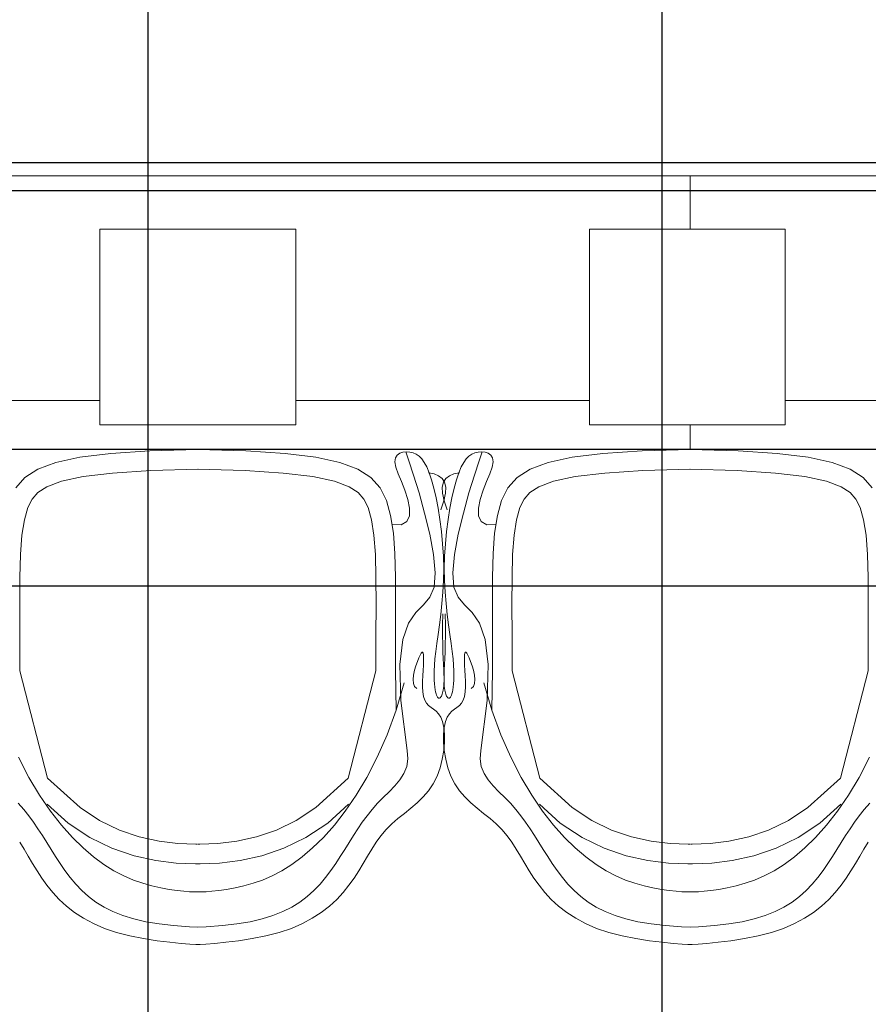
# Model space of a CAD drawing. Units: inches. Extents: x 1454 to 2136, y 626 to 1213.
# Tile 9 of 23: x 1620 to 1654, y 1062 to 1101. Entities that reach past the tile are written whole.
import ezdxf

# ---------------------------------------------------------------- set-up
doc = ezdxf.new("R2010")
doc.units = ezdxf.units.IN
doc.header["$MEASUREMENT"] = 0
for name, color, linetype, lineweight in [('A-ANNO-DIMS', 2, 'Continuous', 18), ('A-FURN-PATT', 252, 'Continuous', 13), ('conference', 41, 'Continuous', 18)]:
    doc.layers.add(name, color=color, linetype=linetype, lineweight=lineweight)
doc.styles.get("Standard").update_dxf_attribs({"font": 'arial.ttf'})
doc.dimstyles.get("Standard").update_dxf_attribs({"dimtxt": 4, "dimasz": 0.18, "dimexe": 0.18, "dimexo": 0.0625, "dimgap": 0.09, "dimtad": 0, "dimtih": 1, "dimtoh": 1, "dimdec": 0, "dimrnd": 6, "dimzin": 0, "dimdsep": 46, "dimlunit": 3, "dimtxsty": 'Standard', "dimcen": 0.09, "dimadec": 0, "dimazin": 0, "dimtfac": 1, "dimtdec": 0, "dimtofl": 0, "dimtmove": 0, "dimatfit": 3, "dimfxl": 1, "dimtolj": 1, "dimtzin": 0, "dimarcsym": 0})

# ---------------------------------------------------------------- blocks, each defined once
blk = doc.blocks.new('ОГ52_на12персон_стол2800х900')
for p, q in [((-1220.7, -341.4), (1220.7, -341.4)), ((-0.6, -341.4), (-0.6, -395.7)), ((-603.4, -595.7), (-603.4, -395.7)), ((-603.4, -395.7), (-403.4, -395.7)), ((-403.4, -395.7), (-403.4, -595.7)), ((-103.4, -595.7), (-103.4, -395.7)), ((-103.4, -395.7), (96.6, -395.7)), ((96.6, -395.7), (96.6, -595.7)), ((-903.4, -570.7), (-603.4, -570.7)), ((-403.4, -570.7), (-103.4, -570.7)), ((96.6, -570.7), (403.4, -570.7)), ((-403.4, -595.7), (-603.4, -595.7)), ((96.6, -595.7), (-103.4, -595.7)), ((-0.6, -595.7), (-0.6, -620.7)), ((-1300, -620.7), (1300, -620.7)), ((-592.3, -624.8), (-552.5, -622.2)), ((-552.5, -622.2), (-503.4, -620.7)), ((-454.3, -622.2), (-503.4, -620.7)), ((-414.4, -624.8), (-454.3, -622.2)), ((-293.9, -623.5), (-290.4, -623.2)), ((-287.8, -632.3), (-290.9, -623.2)), ((-290.4, -623.2), (-286.9, -623.5)), ((-213.6, -623.2), (-217.1, -623.5)), ((-216.2, -632.3), (-213.1, -623.2)), ((-210.1, -623.5), (-213.6, -623.2)), ((-89.6, -624.8), (-49.7, -622.2)), ((-49.7, -622.2), (-0.6, -620.7)), ((48.5, -622.2), (-0.6, -620.7)), ((88.3, -624.8), (48.5, -622.2)), ((-648.5, -633.9), (-624, -628.7)), ((-624, -628.7), (-592.3, -624.8)), ((-382.8, -628.7), (-414.4, -624.8)), ((-358.3, -633.9), (-382.8, -628.7)), ((-302.1, -633.5), (-301.5, -629.4)), ((-301.5, -629.4), (-299.7, -626.5)), ((-299.7, -626.5), (-297.1, -624.6)), ((-297.1, -624.6), (-293.9, -623.5)), ((-283.1, -646.8), (-287.8, -632.3)), ((-286.9, -623.5), (-283.6, -624.2)), ((-283.6, -624.2), (-280.4, -625.5)), ((-280.4, -625.5), (-277.5, -627.4)), ((-277.5, -627.4), (-274.7, -630.2)), ((-274.7, -630.2), (-272.1, -633.9)), ((-229.3, -630.2), (-231.9, -633.9)), ((-226.5, -627.4), (-229.3, -630.2)), ((-223.6, -625.5), (-226.5, -627.4)), ((-220.4, -624.2), (-223.6, -625.5)), ((-220.9, -646.8), (-216.2, -632.3)), ((-217.1, -623.5), (-220.4, -624.2)), ((-206.9, -624.6), (-210.1, -623.5)), ((-204.3, -626.5), (-206.9, -624.6)), ((-202.5, -629.4), (-204.3, -626.5)), ((-201.9, -633.5), (-202.5, -629.4)), ((-145.7, -633.9), (-121.2, -628.7)), ((-121.2, -628.7), (-89.6, -624.8)), ((120, -628.7), (88.3, -624.8)), ((144.5, -633.9), (120, -628.7)), ((-680.2, -649.4), (-666.8, -640.7)), ((-666.8, -640.7), (-648.5, -633.9)), ((-590.5, -644.8), (-551.5, -642.2)), ((-551.5, -642.2), (-502.7, -640.7)), ((-455.2, -642.2), (-504, -640.7)), ((-416.3, -644.8), (-455.2, -642.2)), ((-339.9, -640.7), (-358.3, -633.9)), ((-326.6, -649.4), (-339.9, -640.7)), ((-301.3, -638.8), (-302.1, -633.5)), ((-298.9, -645.6), (-301.3, -638.8)), ((-272.1, -633.9), (-269.5, -638.6)), ((-269.5, -638.6), (-267.1, -644.5)), ((-234.5, -638.6), (-236.9, -644.5)), ((-231.9, -633.9), (-234.5, -638.6)), ((-205.1, -645.6), (-202.7, -638.8)), ((-202.7, -638.8), (-201.9, -633.5)), ((-177.4, -649.4), (-164.1, -640.7)), ((-164.1, -640.7), (-145.7, -633.9)), ((-87.8, -644.8), (-48.8, -642.2)), ((-48.8, -642.2), (0, -640.7)), ((47.5, -642.2), (-1.3, -640.7)), ((86.5, -644.8), (47.5, -642.2)), ((162.8, -640.7), (144.5, -633.9)), ((176.2, -649.4), (162.8, -640.7)), ((-689.5, -660), (-680.2, -649.4)), ((-657.8, -658.7), (-642.8, -653.1)), ((-642.8, -653.1), (-620.7, -648.4)), ((-620.7, -648.4), (-590.5, -644.8)), ((-386.1, -648.4), (-416.3, -644.8)), ((-363.9, -653.1), (-386.1, -648.4)), ((-349, -658.7), (-363.9, -653.1)), ((-317.3, -660), (-326.6, -649.4)), ((-298.9, -645.6), (-295.5, -653.4)), ((-295.5, -653.4), (-292, -662.3)), ((-277.5, -665.1), (-283.1, -646.8)), ((-262.2, -645.6), (-267.7, -644.5)), ((-267.1, -644.5), (-264.7, -651.7)), ((-264.7, -651.7), (-262.3, -660.3)), ((-257.6, -647.6), (-262.2, -645.6)), ((-254, -650.4), (-257.6, -647.6)), ((-251.5, -654.2), (-254, -650.4)), ((-252.5, -654.2), (-250, -650.4)), ((-250, -650.4), (-246.4, -647.6)), ((-246.4, -647.6), (-241.8, -645.6)), ((-241.8, -645.6), (-236.3, -644.5)), ((-239.3, -651.7), (-241.7, -660.3)), ((-236.9, -644.5), (-239.3, -651.7)), ((-226.5, -665.1), (-220.9, -646.8)), ((-208.5, -653.4), (-212, -662.3)), ((-205.1, -645.6), (-208.5, -653.4)), ((-186.7, -660), (-177.4, -649.4)), ((-155.1, -658.7), (-140.1, -653.1)), ((-140.1, -653.1), (-117.9, -648.4)), ((-117.9, -648.4), (-87.8, -644.8)), ((116.7, -648.4), (86.5, -644.8)), ((138.8, -653.1), (116.7, -648.4)), ((153.8, -658.7), (138.8, -653.1)), ((185.5, -660), (176.2, -649.4)), ((-666.9, -664.7), (-657.8, -658.7)), ((-339.8, -664.7), (-349, -658.7)), ((-310.9, -672.9), (-317.3, -660)), ((-292, -662.3), (-289.1, -671.7)), ((-262.3, -660.3), (-260.1, -670)), ((-253.8, -659.2), (-252.5, -654.2)), ((-253.6, -665.5), (-253.8, -659.2)), ((-250.2, -659.2), (-251.5, -654.2)), ((-250.4, -665.5), (-250.2, -659.2)), ((-241.7, -660.3), (-243.9, -670)), ((-212, -662.3), (-214.9, -671.7)), ((-193.1, -672.9), (-186.7, -660)), ((-164.2, -664.7), (-155.1, -658.7)), ((162.9, -664.7), (153.8, -658.7)), ((-677.1, -680.1), (-672.7, -671.3)), ((-672.7, -671.3), (-666.9, -664.7)), ((-334, -671.3), (-339.8, -664.7)), ((-329.6, -680.1), (-334, -671.3)), ((-306.5, -688.1), (-310.9, -672.9)), ((-289.1, -671.7), (-287.3, -680.7)), ((-271.8, -685.8), (-277.5, -665.1)), ((-260.1, -670), (-258, -680.8)), ((-255.4, -682.4), (-252.1, -673.2)), ((-251.9, -673.2), (-253.6, -665.5)), ((-252.1, -673.2), (-250.4, -665.5)), ((-248.6, -682.4), (-251.9, -673.2)), ((-243.9, -670), (-246, -680.8)), ((-232.2, -685.8), (-226.5, -665.1)), ((-214.9, -671.7), (-216.7, -680.7)), ((-197.5, -688.1), (-193.1, -672.9)), ((-174.4, -680.1), (-170, -671.3)), ((-170, -671.3), (-164.2, -664.7)), ((168.7, -671.3), (162.9, -664.7)), ((173.1, -680.1), (168.7, -671.3)), ((-680.6, -692.4), (-677.1, -680.1)), ((-326.1, -692.4), (-329.6, -680.1)), ((-287.3, -680.7), (-287.3, -688.5)), ((-258, -680.8), (-256.2, -692.3)), ((-246, -680.8), (-247.8, -692.3)), ((-216.7, -680.7), (-216.7, -688.5)), ((-177.9, -692.4), (-174.4, -680.1)), ((176.6, -692.4), (173.1, -680.1)), ((-683.1, -708.3), (-680.6, -692.4)), ((-323.6, -708.3), (-326.1, -692.4)), ((-303.7, -706), (-306.5, -688.1)), ((-287.3, -688.5), (-289.9, -694.3)), ((-266.6, -707.3), (-271.8, -685.8)), ((-256.2, -692.3), (-254.6, -704.4)), ((-247.8, -692.3), (-249.4, -704.4)), ((-237.4, -707.3), (-232.2, -685.8)), ((-216.7, -688.5), (-214.1, -694.3)), ((-200.3, -706), (-197.5, -688.1)), ((-180.4, -708.3), (-177.9, -692.4)), ((179.1, -708.3), (176.6, -692.4)), ((-295.6, -697.5), (-305.1, -697.1)), ((-289.9, -694.3), (-295.6, -697.5)), ((-214.1, -694.3), (-208.4, -697.5)), ((-208.4, -697.5), (-198.9, -697.1)), ((-684.6, -728), (-683.1, -708.3)), ((-322.1, -728), (-323.6, -708.3)), ((-302.2, -726.9), (-303.7, -706)), ((-262.8, -728.1), (-266.6, -707.3)), ((-254.6, -704.4), (-253.4, -716.9)), ((-249.4, -704.4), (-250.6, -716.9)), ((-241.2, -728.1), (-237.4, -707.3)), ((-201.8, -726.9), (-200.3, -706)), ((-181.9, -728), (-180.4, -708.3)), ((180.6, -728), (179.1, -708.3)), ((-253.4, -716.9), (-252.6, -729.5)), ((-250.6, -716.9), (-251.4, -729.5)), ((-685.3, -751.4), (-684.6, -728)), ((-321.5, -751.4), (-322.1, -728)), ((-301.5, -751.1), (-302.2, -726.9)), ((-261.1, -746.6), (-262.8, -728.1)), ((-252.6, -729.5), (-252.3, -742.1)), ((-251.4, -729.5), (-251.7, -742.1)), ((-242.9, -746.6), (-241.2, -728.1)), ((-202.5, -751.1), (-201.8, -726.9)), ((-182.5, -751.4), (-181.9, -728)), ((181.2, -751.4), (180.6, -728)), ((-252.3, -742.1), (-252.5, -754.5)), ((-251.7, -742.1), (-251.5, -754.5)), ((-685.4, -778.9), (-685.3, -751.4)), ((-321.4, -778.9), (-321.5, -751.4)), ((-301.4, -778.9), (-301.5, -751.1)), ((-262.2, -761.4), (-261.1, -746.6)), ((-241.8, -761.4), (-242.9, -746.6)), ((-202.6, -778.9), (-202.5, -751.1)), ((-182.6, -778.9), (-182.5, -751.4)), ((181.4, -778.9), (181.2, -751.4)), ((-266.5, -771.5), (-262.2, -761.4)), ((-252.5, -754.5), (-253.1, -766.5)), ((-251.5, -754.5), (-250.9, -766.5)), ((-237.5, -771.5), (-241.8, -761.4)), ((-273.1, -779.2), (-266.5, -771.5)), ((-253.1, -766.5), (-254.1, -778.1)), ((-250.9, -766.5), (-249.9, -778.1)), ((-230.9, -779.2), (-237.5, -771.5)), ((-685.3, -810.5), (-685.4, -778.9)), ((-321.5, -810.5), (-321.4, -778.9)), ((-301.5, -810.6), (-301.4, -778.9)), ((-280.7, -787), (-273.1, -779.2)), ((-254.1, -778.1), (-255.4, -789.2)), ((-249.9, -778.1), (-248.7, -789.2)), ((-223.3, -787), (-230.9, -779.2)), ((-202.5, -810.6), (-202.6, -778.9)), ((-182.5, -810.5), (-182.6, -778.9)), ((181.3, -810.5), (181.4, -778.9)), ((-288.1, -798), (-280.7, -787)), ((-255.4, -789.2), (-256.7, -799.7)), ((-253.5, -800.2), (-253.3, -788.5)), ((-250.5, -800.2), (-250.7, -788.5)), ((-248.7, -789.2), (-247.3, -799.7)), ((-215.9, -798), (-223.3, -787)), ((-294, -814.7), (-288.1, -798)), ((-256.7, -799.7), (-258, -809.6)), ((-253.4, -810.5), (-253.5, -800.2)), ((-250.6, -810.5), (-250.5, -800.2)), ((-247.3, -799.7), (-246, -809.6)), ((-210.1, -814.7), (-215.9, -798)), ((-685.3, -846.6), (-685.3, -810.5)), ((-321.5, -846.6), (-321.5, -810.5)), ((-301.5, -846.4), (-301.5, -810.6)), ((-258, -809.6), (-259.3, -818.7)), ((-253.3, -819.6), (-253.4, -810.5)), ((-250.7, -819.6), (-250.6, -810.5)), ((-246, -809.6), (-244.7, -818.7)), ((-202.5, -846.4), (-202.5, -810.6)), ((-182.5, -846.6), (-182.5, -810.5)), ((181.3, -846.6), (181.3, -810.5)), ((-297, -840.1), (-294, -814.7)), ((-259.3, -818.7), (-260.4, -827)), ((-253.1, -827.5), (-253.3, -819.6)), ((-250.9, -827.5), (-250.7, -819.6)), ((-244.7, -818.7), (-243.6, -827)), ((-207, -840.1), (-210.1, -814.7)), ((-279.2, -837.1), (-277.7, -833.4)), ((-277.7, -833.4), (-276.4, -830.6)), ((-276.4, -830.6), (-275.3, -828.7)), ((-275.3, -828.7), (-274.4, -827.8)), ((-274.4, -827.8), (-273.8, -827.7)), ((-273.8, -827.7), (-273.3, -828.6)), ((-273.3, -828.6), (-272.9, -830.5)), ((-272.9, -830.5), (-272.8, -833.2)), ((-272.8, -833.2), (-272.9, -836.7)), ((-260.4, -827), (-261.2, -834.4)), ((-252.8, -834.3), (-253.1, -827.5)), ((-252.5, -840.3), (-252.8, -834.3)), ((-251.5, -840.3), (-251.2, -834.3)), ((-251.2, -834.3), (-250.9, -827.5)), ((-243.6, -827), (-242.8, -834.4)), ((-231.1, -830.5), (-231.2, -833.2)), ((-231.2, -833.2), (-231.1, -836.7)), ((-230.7, -828.6), (-231.1, -830.5)), ((-230.3, -827.7), (-230.7, -828.6)), ((-229.6, -827.8), (-230.3, -827.7)), ((-228.7, -828.7), (-229.6, -827.8)), ((-227.6, -830.6), (-228.7, -828.7)), ((-226.3, -833.4), (-227.6, -830.6)), ((-224.8, -837.1), (-226.3, -833.4)), ((-296, -876.9), (-297, -840.1)), ((-282, -846.2), (-280.7, -841.5)), ((-280.7, -841.5), (-279.2, -837.1)), ((-273.1, -841.2), (-273.4, -846.2)), ((-272.9, -836.7), (-273.1, -841.2)), ((-261.7, -841), (-262, -846.8)), ((-261.2, -834.4), (-261.7, -841)), ((-252.3, -845.4), (-252.5, -840.3)), ((-251.7, -845.4), (-251.5, -840.3)), ((-242.8, -834.4), (-242.3, -841)), ((-242.3, -841), (-242, -846.8)), ((-231.1, -836.7), (-230.9, -841.2)), ((-230.9, -841.2), (-230.6, -846.2)), ((-223.3, -841.5), (-224.8, -837.1)), ((-222, -846.2), (-223.3, -841.5)), ((-208, -876.9), (-207, -840.1)), ((-657, -956.4), (-685.3, -846.6)), ((-349.8, -956.4), (-321.5, -846.6)), ((-301, -886.8), (-301.5, -846.4)), ((-283.5, -855.5), (-283, -851)), ((-283, -851), (-282, -846.2)), ((-273.6, -851.7), (-273.8, -857.3)), ((-273.4, -846.2), (-273.6, -851.7)), ((-262, -846.8), (-262, -851.9)), ((-262, -851.9), (-261.9, -856.3)), ((-252.1, -849.8), (-252.3, -845.4)), ((-252, -853.7), (-252.1, -849.8)), ((-252, -853.7), (-251.9, -849.8)), ((-252, -857), (-252, -853.7)), ((-252, -857), (-252, -853.7)), ((-251.9, -849.8), (-251.7, -845.4)), ((-242, -851.9), (-242.1, -856.3)), ((-242, -846.8), (-242, -851.9)), ((-230.6, -846.2), (-230.4, -851.7)), ((-230.4, -851.7), (-230.2, -857.3)), ((-221, -851), (-222, -846.2)), ((-220.5, -855.5), (-221, -851)), ((-203, -886.8), (-202.5, -846.4)), ((-154.2, -956.4), (-182.5, -846.6)), ((153, -956.4), (181.3, -846.6)), ((-292.7, -859), (-301, -886.8)), ((-283.2, -859.6), (-283.5, -855.5)), ((-282.1, -862.7), (-283.2, -859.6)), ((-279.9, -864.8), (-282.1, -862.7)), ((-273.8, -857.3), (-273.8, -862.9)), ((-273.8, -862.9), (-273.5, -868.2)), ((-261.9, -856.3), (-261.7, -860.1)), ((-261.7, -860.1), (-261.4, -863.3)), ((-261.4, -863.3), (-261, -866)), ((-252.8, -866.3), (-252.5, -864.5)), ((-252.5, -864.5), (-252.3, -862.4)), ((-252.3, -862.4), (-252.1, -859.9)), ((-252.1, -859.9), (-252, -857)), ((-251.9, -859.9), (-252, -857)), ((-251.7, -862.4), (-251.9, -859.9)), ((-251.5, -864.5), (-251.7, -862.4)), ((-251.2, -866.3), (-251.5, -864.5)), ((-242.6, -863.3), (-243, -866)), ((-242.3, -860.1), (-242.6, -863.3)), ((-242.1, -856.3), (-242.3, -860.1)), ((-230.2, -862.9), (-230.5, -868.2)), ((-230.2, -857.3), (-230.2, -862.9)), ((-224.1, -864.8), (-221.9, -862.7)), ((-221.9, -862.7), (-220.8, -859.6)), ((-220.8, -859.6), (-220.5, -855.5)), ((-211.3, -859), (-203, -886.8)), ((-273.5, -868.2), (-272.8, -872.9)), ((-272.8, -872.9), (-271.6, -876.8)), ((-261, -866), (-260.6, -868.3)), ((-260.6, -868.3), (-260.1, -870.2)), ((-260.1, -870.2), (-259.6, -871.7)), ((-259.6, -871.7), (-259.1, -872.9)), ((-259.1, -872.9), (-258.6, -873.7)), ((-258.6, -873.7), (-258.1, -874.3)), ((-258.1, -874.3), (-257.6, -874.6)), ((-256.5, -874.6), (-256, -874.3)), ((-256, -874.3), (-255.6, -873.9)), ((-255.6, -873.9), (-255.1, -873.3)), ((-255.1, -873.3), (-254.7, -872.5)), ((-254.7, -872.5), (-254.2, -871.6)), ((-254.2, -871.6), (-253.8, -870.5)), ((-253.8, -870.5), (-253.5, -869.2)), ((-253.5, -869.2), (-253.1, -867.9)), ((-253.1, -867.9), (-252.8, -866.3)), ((-250.9, -867.9), (-251.2, -866.3)), ((-250.6, -869.2), (-250.9, -867.9)), ((-250.2, -870.5), (-250.6, -869.2)), ((-249.8, -871.6), (-250.2, -870.5)), ((-249.3, -872.5), (-249.8, -871.6)), ((-248.9, -873.3), (-249.3, -872.5)), ((-248.4, -873.9), (-248.9, -873.3)), ((-248, -874.3), (-248.4, -873.9)), ((-247.5, -874.6), (-248, -874.3)), ((-245.9, -874.3), (-246.4, -874.6)), ((-245.4, -873.7), (-245.9, -874.3)), ((-244.9, -872.9), (-245.4, -873.7)), ((-244.4, -871.7), (-244.9, -872.9)), ((-243.9, -870.2), (-244.4, -871.7)), ((-243.4, -868.3), (-243.9, -870.2)), ((-243, -866), (-243.4, -868.3)), ((-231.2, -872.9), (-232.4, -876.8)), ((-230.5, -868.2), (-231.2, -872.9)), ((-289.6, -927.9), (-296, -876.9)), ((-271.6, -876.8), (-269.8, -879.9)), ((-269.8, -879.9), (-267.7, -882.2)), ((-267.7, -882.2), (-265.2, -884.1)), ((-265.2, -884.1), (-262.6, -886)), ((-257.6, -874.6), (-257, -874.7)), ((-257, -874.7), (-256.5, -874.6)), ((-247, -874.7), (-247.5, -874.6)), ((-246.4, -874.6), (-247, -874.7)), ((-238.8, -884.1), (-241.4, -886)), ((-236.3, -882.2), (-238.8, -884.1)), ((-234.2, -879.9), (-236.3, -882.2)), ((-232.4, -876.8), (-234.2, -879.9)), ((-214.4, -927.9), (-208, -876.9)), ((-301, -886.8), (-310.2, -912.1)), ((-262.6, -886), (-260, -888)), ((-260, -888), (-257.5, -890.6)), ((-257.5, -890.6), (-255.3, -894)), ((-255.3, -894), (-253.5, -898.6)), ((-248.7, -894), (-250.5, -898.6)), ((-246.5, -890.6), (-248.7, -894)), ((-244, -888), (-246.5, -890.6)), ((-241.4, -886), (-244, -888)), ((-203, -886.8), (-193.8, -912.1)), ((-253.5, -898.6), (-252.3, -904.5)), ((-251.7, -904.5), (-252.4, -911.6)), ((-252.3, -904.5), (-251.6, -911.6)), ((-250.5, -898.6), (-251.7, -904.5)), ((-310.2, -912.1), (-320.1, -934.9)), ((-252.4, -911.6), (-252.4, -919.5)), ((-251.6, -911.6), (-251.6, -919.5)), ((-193.8, -912.1), (-183.9, -934.9)), ((-252.4, -919.5), (-251.7, -928)), ((-251.6, -919.5), (-252.3, -928)), ((-289.6, -927.9), (-288.8, -936.5)), ((-252.3, -928), (-253.8, -936.8)), ((-251.7, -928), (-250.2, -936.8)), ((-214.4, -927.9), (-215.2, -936.5)), ((-686.6, -934.9), (-676.1, -955.5)), ((-320.1, -934.9), (-330.7, -955.5)), ((-290, -944.3), (-292.9, -951.4)), ((-288.8, -936.5), (-290, -944.3)), ((-253.8, -936.8), (-256, -945.6)), ((-250.2, -936.8), (-248, -945.6)), ((-215.2, -936.5), (-214, -944.3)), ((-214, -944.3), (-211.1, -951.4)), ((-183.9, -934.9), (-173.3, -955.5)), ((182.6, -934.9), (172.1, -955.5)), ((-292.9, -951.4), (-297.1, -958)), ((-259.1, -954.1), (-263, -962)), ((-256, -945.6), (-259.1, -954.1)), ((-248, -945.6), (-244.9, -954.1)), ((-244.9, -954.1), (-241, -962)), ((-211.1, -951.4), (-206.9, -958)), ((-676.1, -955.5), (-665.2, -973.8)), ((-657, -956.4), (-623.7, -986.3)), ((-349.8, -956.4), (-383, -986.3)), ((-330.7, -955.5), (-341.6, -973.8)), ((-302.3, -964.1), (-308, -970.1)), ((-297.1, -958), (-302.3, -964.1)), ((-263, -962), (-267.8, -969.1)), ((-241, -962), (-236.2, -969.1)), ((-206.9, -958), (-201.7, -964.1)), ((-201.7, -964.1), (-196, -970.1)), ((-173.3, -955.5), (-162.4, -973.8)), ((-154.2, -956.4), (-121, -986.3)), ((153, -956.4), (119.7, -986.3)), ((172.1, -955.5), (161.2, -973.8)), ((-665.2, -973.8), (-654, -990)), ((-341.6, -973.8), (-352.8, -990)), ((-308, -970.1), (-314.1, -976)), ((-267.8, -969.1), (-273.4, -975.5)), ((-236.2, -969.1), (-230.6, -975.5)), ((-196, -970.1), (-190, -976)), ((-162.4, -973.8), (-151.3, -990)), ((161.2, -973.8), (150, -990)), ((-686.8, -982), (-681.3, -988.2)), ((-657.3, -983), (-636, -1002.1)), ((-349.4, -983), (-370.7, -1002.1)), ((-320, -982), (-325.5, -988.2)), ((-314.1, -976), (-320, -982)), ((-279.5, -981.4), (-285.9, -986.9)), ((-273.4, -975.5), (-279.5, -981.4)), ((-230.6, -975.5), (-224.5, -981.4)), ((-224.5, -981.4), (-218.1, -986.9)), ((-190, -976), (-184, -982)), ((-184, -982), (-178.5, -988.2)), ((-154.6, -983), (-133.3, -1002.1)), ((153.3, -983), (132, -1002.1)), ((182.8, -982), (177.3, -988.2)), ((-681.3, -988.2), (-676.1, -994.6)), ((-676.1, -994.6), (-671.3, -1001.3)), ((-654, -990), (-642.7, -1004.3)), ((-623.7, -986.3), (-603.8, -999.5)), ((-383, -986.3), (-402.9, -999.5)), ((-352.8, -990), (-364, -1004.3)), ((-330.6, -994.6), (-335.5, -1001.3)), ((-325.5, -988.2), (-330.6, -994.6)), ((-292.5, -992.3), (-299, -997.6)), ((-285.9, -986.9), (-292.5, -992.3)), ((-218.1, -986.9), (-211.5, -992.3)), ((-211.5, -992.3), (-205, -997.6)), ((-178.5, -988.2), (-173.4, -994.6)), ((-173.4, -994.6), (-168.6, -1001.3)), ((-151.3, -990), (-140, -1004.3)), ((-121, -986.3), (-101.1, -999.5)), ((119.7, -986.3), (99.8, -999.5)), ((150, -990), (138.7, -1004.3)), ((172.1, -994.6), (167.3, -1001.3)), ((177.3, -988.2), (172.1, -994.6)), ((-671.3, -1001.3), (-666.7, -1008.1)), ((-642.7, -1004.3), (-631.5, -1016.8)), ((-636, -1002.1), (-613.8, -1016.9)), ((-603.8, -999.5), (-583.6, -1009.3)), ((-402.9, -999.5), (-423.2, -1009.3)), ((-370.7, -1002.1), (-393, -1016.9)), ((-364, -1004.3), (-375.2, -1016.8)), ((-335.5, -1001.3), (-340.1, -1008.1)), ((-305.3, -1003), (-311.2, -1008.8)), ((-299, -997.6), (-305.3, -1003)), ((-205, -997.6), (-198.7, -1003)), ((-198.7, -1003), (-192.8, -1008.8)), ((-168.6, -1001.3), (-163.9, -1008.1)), ((-140, -1004.3), (-128.8, -1016.8)), ((-133.3, -1002.1), (-111, -1016.9)), ((-101.1, -999.5), (-80.8, -1009.3)), ((99.8, -999.5), (79.6, -1009.3)), ((132, -1002.1), (109.8, -1016.9)), ((138.7, -1004.3), (127.5, -1016.8)), ((167.3, -1001.3), (162.7, -1008.1)), ((-666.7, -1008.1), (-662.2, -1015)), ((-662.2, -1015), (-657.8, -1022.1)), ((-583.6, -1009.3), (-563.2, -1016.2)), ((-423.2, -1009.3), (-443.5, -1016.2)), ((-344.5, -1015), (-348.9, -1022.1)), ((-340.1, -1008.1), (-344.5, -1015)), ((-316.5, -1015.1), (-321.3, -1021.7)), ((-311.2, -1008.8), (-316.5, -1015.1)), ((-192.8, -1008.8), (-187.5, -1015.1)), ((-187.5, -1015.1), (-182.7, -1021.7)), ((-163.9, -1008.1), (-159.5, -1015)), ((-159.5, -1015), (-155.1, -1022.1)), ((-80.8, -1009.3), (-60.5, -1016.2)), ((79.6, -1009.3), (59.2, -1016.2)), ((158.2, -1015), (153.8, -1022.1)), ((162.7, -1008.1), (158.2, -1015)), ((-685.4, -1021.7), (-680.9, -1028.7)), ((-657.8, -1022.1), (-653.4, -1029.2)), ((-631.5, -1016.8), (-620.6, -1027.5)), ((-613.8, -1016.9), (-591.2, -1027.9)), ((-563.2, -1016.2), (-543.1, -1020.6)), ((-543.1, -1020.6), (-523.8, -1023)), ((-523.8, -1023), (-505.5, -1023.8)), ((-505.5, -1023.8), (-503.8, -1023.8)), ((-501.3, -1023.8), (-503, -1023.8)), ((-483, -1023), (-501.3, -1023.8)), ((-463.6, -1020.6), (-483, -1023)), ((-443.5, -1016.2), (-463.6, -1020.6)), ((-393, -1016.9), (-415.6, -1027.9)), ((-375.2, -1016.8), (-386.2, -1027.5)), ((-348.9, -1022.1), (-353.4, -1029.2)), ((-321.3, -1021.7), (-325.8, -1028.7)), ((-182.7, -1021.7), (-178.2, -1028.7)), ((-155.1, -1022.1), (-150.6, -1029.2)), ((-128.8, -1016.8), (-117.9, -1027.5)), ((-111, -1016.9), (-88.4, -1027.9)), ((-60.5, -1016.2), (-40.4, -1020.6)), ((-40.4, -1020.6), (-21, -1023)), ((-21, -1023), (-2.7, -1023.8)), ((-2.7, -1023.8), (-1, -1023.8)), ((1.5, -1023.8), (-0.2, -1023.8)), ((19.7, -1023), (1.5, -1023.8)), ((39.1, -1020.6), (19.7, -1023)), ((59.2, -1016.2), (39.1, -1020.6)), ((109.8, -1016.9), (87.2, -1027.9)), ((127.5, -1016.8), (116.6, -1027.5)), ((153.8, -1022.1), (149.4, -1029.2)), ((181.4, -1021.7), (176.9, -1028.7)), ((-680.9, -1028.7), (-676.6, -1035.9)), ((-653.4, -1029.2), (-648.8, -1036.4)), ((-620.6, -1027.5), (-609.9, -1036.7)), ((-591.2, -1027.9), (-568.6, -1035.5)), ((-415.6, -1027.9), (-438.1, -1035.5)), ((-386.2, -1027.5), (-396.9, -1036.7)), ((-353.4, -1029.2), (-357.9, -1036.4)), ((-325.8, -1028.7), (-330.2, -1035.9)), ((-178.2, -1028.7), (-173.9, -1035.9)), ((-150.6, -1029.2), (-146.1, -1036.4)), ((-117.9, -1027.5), (-107.1, -1036.7)), ((-88.4, -1027.9), (-65.9, -1035.5)), ((87.2, -1027.9), (64.6, -1035.5)), ((116.6, -1027.5), (105.9, -1036.7)), ((149.4, -1029.2), (144.8, -1036.4)), ((176.9, -1028.7), (172.6, -1035.9)), ((-676.6, -1035.9), (-672.2, -1043.3)), ((-672.2, -1043.3), (-667.7, -1050.8)), ((-648.8, -1036.4), (-644.1, -1043.6)), ((-644.1, -1043.6), (-639.2, -1050.7)), ((-609.9, -1036.7), (-599.4, -1044.4)), ((-599.4, -1044.4), (-589.1, -1050.8)), ((-568.6, -1035.5), (-546.5, -1040.4)), ((-546.5, -1040.4), (-525.4, -1043)), ((-525.4, -1043), (-505.7, -1043.8)), ((-505.7, -1043.8), (-503.4, -1043.8)), ((-501, -1043.8), (-503.4, -1043.8)), ((-481.3, -1043), (-501, -1043.8)), ((-460.2, -1040.4), (-481.3, -1043)), ((-438.1, -1035.5), (-460.2, -1040.4)), ((-407.4, -1044.4), (-417.6, -1050.8)), ((-396.9, -1036.7), (-407.4, -1044.4)), ((-362.6, -1043.6), (-367.6, -1050.7)), ((-357.9, -1036.4), (-362.6, -1043.6)), ((-334.5, -1043.3), (-339, -1050.8)), ((-330.2, -1035.9), (-334.5, -1043.3)), ((-173.9, -1035.9), (-169.5, -1043.3)), ((-169.5, -1043.3), (-165, -1050.8)), ((-146.1, -1036.4), (-141.4, -1043.6)), ((-141.4, -1043.6), (-136.4, -1050.7)), ((-107.1, -1036.7), (-96.6, -1044.4)), ((-96.6, -1044.4), (-86.4, -1050.8)), ((-65.9, -1035.5), (-43.8, -1040.4)), ((-43.8, -1040.4), (-22.7, -1043)), ((-22.7, -1043), (-3, -1043.8)), ((-3, -1043.8), (-0.6, -1043.8)), ((1.7, -1043.8), (-0.6, -1043.8)), ((21.4, -1043), (1.7, -1043.8)), ((42.5, -1040.4), (21.4, -1043)), ((64.6, -1035.5), (42.5, -1040.4)), ((95.4, -1044.4), (85.1, -1050.8)), ((105.9, -1036.7), (95.4, -1044.4)), ((140.1, -1043.6), (135.2, -1050.7)), ((144.8, -1036.4), (140.1, -1043.6)), ((168.2, -1043.3), (163.7, -1050.8)), ((172.6, -1035.9), (168.2, -1043.3)), ((-667.7, -1050.8), (-662.9, -1058.3)), ((-639.2, -1050.7), (-633.9, -1057.7)), ((-589.1, -1050.8), (-579.1, -1056)), ((-417.6, -1050.8), (-427.6, -1056)), ((-367.6, -1050.7), (-372.9, -1057.7)), ((-339, -1050.8), (-343.8, -1058.3)), ((-165, -1050.8), (-160.2, -1058.3)), ((-136.4, -1050.7), (-131.1, -1057.7)), ((-86.4, -1050.8), (-76.4, -1056)), ((85.1, -1050.8), (75.1, -1056)), ((135.2, -1050.7), (129.8, -1057.7)), ((163.7, -1050.8), (158.9, -1058.3)), ((-662.9, -1058.3), (-657.6, -1065.7)), ((-633.9, -1057.7), (-628.1, -1064.5)), ((-628.1, -1064.5), (-621.9, -1071)), ((-579.1, -1056), (-569.3, -1060.3)), ((-569.3, -1060.3), (-559.7, -1063.6)), ((-559.7, -1063.6), (-550.4, -1066.3)), ((-447, -1063.6), (-456.3, -1066.3)), ((-437.4, -1060.3), (-447, -1063.6)), ((-427.6, -1056), (-437.4, -1060.3)), ((-378.6, -1064.5), (-384.9, -1071)), ((-372.9, -1057.7), (-378.6, -1064.5)), ((-343.8, -1058.3), (-349.1, -1065.7)), ((-160.2, -1058.3), (-154.9, -1065.7)), ((-131.1, -1057.7), (-125.4, -1064.5)), ((-125.4, -1064.5), (-119.1, -1071)), ((-76.4, -1056), (-66.6, -1060.3)), ((-66.6, -1060.3), (-57, -1063.6)), ((-57, -1063.6), (-47.7, -1066.3)), ((55.7, -1063.6), (46.4, -1066.3)), ((65.3, -1060.3), (55.7, -1063.6)), ((75.1, -1056), (65.3, -1060.3)), ((124.1, -1064.5), (117.9, -1071)), ((129.8, -1057.7), (124.1, -1064.5)), ((158.9, -1058.3), (153.6, -1065.7)), ((-657.6, -1065.7), (-651.7, -1073)), ((-651.7, -1073), (-645.1, -1080.1)), ((-621.9, -1071), (-615, -1077.1)), ((-550.4, -1066.3), (-541.3, -1068.3)), ((-541.3, -1068.3), (-532.7, -1069.9)), ((-532.7, -1069.9), (-524.7, -1071)), ((-524.7, -1071), (-517.7, -1071.7)), ((-517.7, -1071.7), (-511.8, -1072.2)), ((-511.8, -1072.2), (-507.3, -1072.4)), ((-507.3, -1072.4), (-504.4, -1072.5)), ((-504.4, -1072.5), (-503.4, -1072.5)), ((-502.3, -1072.5), (-503.4, -1072.5)), ((-499.4, -1072.4), (-502.3, -1072.5)), ((-494.9, -1072.2), (-499.4, -1072.4)), ((-489.1, -1071.7), (-494.9, -1072.2)), ((-482, -1071), (-489.1, -1071.7)), ((-474.1, -1069.9), (-482, -1071)), ((-465.4, -1068.3), (-474.1, -1069.9)), ((-456.3, -1066.3), (-465.4, -1068.3)), ((-384.9, -1071), (-391.7, -1077.1)), ((-355, -1073), (-361.6, -1080.1)), ((-349.1, -1065.7), (-355, -1073)), ((-154.9, -1065.7), (-149, -1073)), ((-149, -1073), (-142.4, -1080.1)), ((-119.1, -1071), (-112.3, -1077.1)), ((-47.7, -1066.3), (-38.6, -1068.3)), ((-38.6, -1068.3), (-29.9, -1069.9)), ((-29.9, -1069.9), (-22, -1071)), ((-22, -1071), (-14.9, -1071.7)), ((-14.9, -1071.7), (-9.1, -1072.2)), ((-9.1, -1072.2), (-4.6, -1072.4)), ((-4.6, -1072.4), (-1.7, -1072.5)), ((-1.7, -1072.5), (-0.6, -1072.5)), ((0.4, -1072.5), (-0.6, -1072.5)), ((3.3, -1072.4), (0.4, -1072.5)), ((7.8, -1072.2), (3.3, -1072.4)), ((13.7, -1071.7), (7.8, -1072.2)), ((20.7, -1071), (13.7, -1071.7)), ((28.7, -1069.9), (20.7, -1071)), ((37.3, -1068.3), (28.7, -1069.9)), ((46.4, -1066.3), (37.3, -1068.3)), ((117.9, -1071), (111, -1077.1)), ((147.7, -1073), (141.1, -1080.1)), ((153.6, -1065.7), (147.7, -1073)), ((-645.1, -1080.1), (-637.7, -1086.9)), ((-615, -1077.1), (-607.5, -1082.8)), ((-607.5, -1082.8), (-599.2, -1088)), ((-399.2, -1082.8), (-407.5, -1088)), ((-391.7, -1077.1), (-399.2, -1082.8)), ((-361.6, -1080.1), (-369, -1086.9)), ((-142.4, -1080.1), (-135, -1086.9)), ((-112.3, -1077.1), (-104.8, -1082.8)), ((-104.8, -1082.8), (-96.5, -1088)), ((103.5, -1082.8), (95.2, -1088)), ((111, -1077.1), (103.5, -1082.8)), ((141.1, -1080.1), (133.7, -1086.9)), ((-637.7, -1086.9), (-629.5, -1093.3)), ((-629.5, -1093.3), (-620.3, -1099.3)), ((-599.2, -1088), (-590.1, -1092.6)), ((-590.1, -1092.6), (-580, -1096.6)), ((-416.6, -1092.6), (-426.7, -1096.6)), ((-407.5, -1088), (-416.6, -1092.6)), ((-377.3, -1093.3), (-386.5, -1099.3)), ((-369, -1086.9), (-377.3, -1093.3)), ((-135, -1086.9), (-126.7, -1093.3)), ((-126.7, -1093.3), (-117.5, -1099.3)), ((-96.5, -1088), (-87.4, -1092.6)), ((-87.4, -1092.6), (-77.3, -1096.6)), ((86.1, -1092.6), (76, -1096.6)), ((95.2, -1088), (86.1, -1092.6)), ((125.5, -1093.3), (116.3, -1099.3)), ((133.7, -1086.9), (125.5, -1093.3)), ((-620.3, -1099.3), (-610.1, -1104.8)), ((-610.1, -1104.8), (-598.8, -1109.7)), ((-580, -1096.6), (-568.9, -1100)), ((-568.9, -1100), (-556.7, -1102.9)), ((-556.7, -1102.9), (-543.1, -1105.2)), ((-543.1, -1105.2), (-528.3, -1106.9)), ((-463.6, -1105.2), (-478.4, -1106.9)), ((-450.1, -1102.9), (-463.6, -1105.2)), ((-437.8, -1100), (-450.1, -1102.9)), ((-426.7, -1096.6), (-437.8, -1100)), ((-396.6, -1104.8), (-407.9, -1109.7)), ((-386.5, -1099.3), (-396.6, -1104.8)), ((-117.5, -1099.3), (-107.4, -1104.8)), ((-107.4, -1104.8), (-96.1, -1109.7)), ((-77.3, -1096.6), (-66.2, -1100)), ((-66.2, -1100), (-53.9, -1102.9)), ((-53.9, -1102.9), (-40.4, -1105.2)), ((-40.4, -1105.2), (-25.6, -1106.9)), ((39.1, -1105.2), (24.3, -1106.9)), ((52.7, -1102.9), (39.1, -1105.2)), ((64.9, -1100), (52.7, -1102.9)), ((76, -1096.6), (64.9, -1100)), ((106.1, -1104.8), (94.8, -1109.7)), ((116.3, -1099.3), (106.1, -1104.8)), ((-598.8, -1109.7), (-586.4, -1113.9)), ((-586.4, -1113.9), (-572.8, -1117.3)), ((-528.3, -1106.9), (-512, -1108.1)), ((-512, -1108.1), (-503.4, -1108.4)), ((-494.8, -1108.1), (-503.4, -1108.4)), ((-478.4, -1106.9), (-494.8, -1108.1)), ((-420.4, -1113.9), (-433.9, -1117.3)), ((-407.9, -1109.7), (-420.4, -1113.9)), ((-96.1, -1109.7), (-83.6, -1113.9)), ((-83.6, -1113.9), (-70.1, -1117.3)), ((-25.6, -1106.9), (-9.3, -1108.1)), ((-9.3, -1108.1), (-0.6, -1108.4)), ((8, -1108.1), (-0.6, -1108.4)), ((24.3, -1106.9), (8, -1108.1)), ((82.4, -1113.9), (68.8, -1117.3)), ((94.8, -1109.7), (82.4, -1113.9)), ((-572.8, -1117.3), (-558.8, -1120.1)), ((-558.8, -1120.1), (-544.9, -1122.3)), ((-544.9, -1122.3), (-531.9, -1123.9)), ((-531.9, -1123.9), (-520.6, -1125.1)), ((-520.6, -1125.1), (-511.5, -1125.8)), ((-511.5, -1125.8), (-505.6, -1126.2)), ((-495.2, -1125.8), (-501.2, -1126.2)), ((-486.2, -1125.1), (-495.2, -1125.8)), ((-474.8, -1123.9), (-486.2, -1125.1)), ((-461.8, -1122.3), (-474.8, -1123.9)), ((-448, -1120.1), (-461.8, -1122.3)), ((-433.9, -1117.3), (-448, -1120.1)), ((-70.1, -1117.3), (-56, -1120.1)), ((-56, -1120.1), (-42.2, -1122.3)), ((-42.2, -1122.3), (-29.2, -1123.9)), ((-29.2, -1123.9), (-17.8, -1125.1)), ((-17.8, -1125.1), (-8.8, -1125.8)), ((-8.8, -1125.8), (-2.8, -1126.2)), ((7.5, -1125.8), (1.6, -1126.2)), ((16.6, -1125.1), (7.5, -1125.8)), ((27.9, -1123.9), (16.6, -1125.1)), ((40.9, -1122.3), (27.9, -1123.9)), ((54.8, -1120.1), (40.9, -1122.3)), ((68.8, -1117.3), (54.8, -1120.1)), ((-505.6, -1126.2), (-503.4, -1126.3)), ((-501.2, -1126.2), (-503.4, -1126.3)), ((-2.8, -1126.2), (-0.6, -1126.3)), ((1.6, -1126.2), (-0.6, -1126.3))]:
    blk.add_line(p, q)
blk = doc.blocks.new('*D33')
at = {"layer": 'A-ANNO-DIMS', "color": 0, "lineweight": -2, "transparency": 16777216}
for p, q in [((2032.494, 1126.282), (1462.374, 1126.282)), ((1462.554, 1126.102), (1462.554, 1056.381)), ((1462.554, 982.462), (1462.554, 1052.184)), ((2032.494, 982.282), (1462.374, 982.282))]:
    blk.add_line(p, q, dxfattribs=at)
at = {"layer": 'A-ANNO-DIMS', "color": 0, "transparency": 16777216}
for points in [[(1462.524, 1126.102), (1462.584, 1126.102), (1462.554, 1126.282)], [(1462.524, 982.462), (1462.584, 982.462), (1462.554, 982.282)]]:
    blk.add_solid(points, dxfattribs=at)
at = {"layer": 'Defpoints', "color": 0, "transparency": 16777216}
for p in [(1462.554, 1126.282), (2032.556, 1126.282), (2032.556, 982.282)]:
    blk.add_point(p, dxfattribs=at)
at = {"layer": 'A-ANNO-DIMS', "color": 0, "transparency": 16777216, "insert": (1462.554, 1054.282), "char_height": 4, "attachment_point": 5}
blk.add_mtext('\\A1;144', dxfattribs=at)
blk = doc.blocks.new('*D40')
at = {"layer": 'A-ANNO-DIMS', "color": 0, "lineweight": -2, "transparency": 16777216}
for p, q in [((1501.556, 877.345), (1501.556, 1210.464)), ((1501.736, 1210.284), (1569.244, 1210.284)), ((1645.376, 1210.284), (1577.869, 1210.284)), ((1645.556, 877.345), (1645.556, 1210.464))]:
    blk.add_line(p, q, dxfattribs=at)
at = {"layer": 'A-ANNO-DIMS', "color": 0, "transparency": 16777216}
for points in [[(1501.736, 1210.314), (1501.736, 1210.254), (1501.556, 1210.284)], [(1645.376, 1210.314), (1645.376, 1210.254), (1645.556, 1210.284)]]:
    blk.add_solid(points, dxfattribs=at)
at = {"layer": 'Defpoints', "color": 0, "transparency": 16777216}
for p in [(1645.556, 1210.284), (1501.556, 877.282), (1645.556, 877.282)]:
    blk.add_point(p, dxfattribs=at)
at = {"layer": 'A-ANNO-DIMS', "color": 0, "transparency": 16777216, "insert": (1573.556, 1210.284), "char_height": 4, "attachment_point": 5}
blk.add_mtext('\\A1;144', dxfattribs=at)
blk = doc.blocks.new('*D54')
at = {"layer": 'A-ANNO-DIMS', "color": 0, "lineweight": -2, "transparency": 16777216}
for p, q in [((1879.494, 1126.282), (1462.374, 1126.282)), ((1462.554, 1126.102), (1462.554, 1078.915)), ((1462.554, 1027.462), (1462.554, 1074.65)), ((1879.494, 1027.282), (1462.374, 1027.282))]:
    blk.add_line(p, q, dxfattribs=at)
at = {"layer": 'A-ANNO-DIMS', "color": 0, "transparency": 16777216}
for points in [[(1462.524, 1126.102), (1462.584, 1126.102), (1462.554, 1126.282)], [(1462.524, 1027.462), (1462.584, 1027.462), (1462.554, 1027.282)]]:
    blk.add_solid(points, dxfattribs=at)
at = {"layer": 'Defpoints', "color": 0, "transparency": 16777216}
for p in [(1879.556, 1126.282), (1462.554, 1027.282), (1879.556, 1027.282)]:
    blk.add_point(p, dxfattribs=at)
at = {"layer": 'A-ANNO-DIMS', "color": 0, "transparency": 16777216, "insert": (1462.554, 1076.782), "char_height": 4, "attachment_point": 5}
blk.add_mtext('\\A1;99', dxfattribs=at)
blk = doc.blocks.new('*D67')
at = {"layer": 'A-ANNO-DIMS', "color": 0, "lineweight": -2, "transparency": 16777216}
for p, q in [((1606.484, 1018.345), (1606.484, 1210.464)), ((1606.664, 1210.284), (1610.595, 1210.284)), ((1624.703, 1210.284), (1620.773, 1210.284)), ((1624.883, 1018.329), (1624.883, 1210.464))]:
    blk.add_line(p, q, dxfattribs=at)
at = {"layer": 'A-ANNO-DIMS', "color": 0, "transparency": 16777216}
for points in [[(1606.664, 1210.314), (1606.664, 1210.254), (1606.484, 1210.284)], [(1624.703, 1210.314), (1624.703, 1210.254), (1624.883, 1210.284)]]:
    blk.add_solid(points, dxfattribs=at)
at = {"layer": 'Defpoints', "color": 0, "transparency": 16777216}
for p in [(1624.883, 1210.284), (1606.484, 1018.282), (1624.883, 1018.267)]:
    blk.add_point(p, dxfattribs=at)
at = {"layer": 'A-ANNO-DIMS', "color": 0, "transparency": 16777216, "insert": (1615.684, 1210.284), "char_height": 4, "attachment_point": 5}
blk.add_mtext('\\A1;18.4', dxfattribs=at)
blk = doc.blocks.new('*D70')
at = {"layer": 'A-ANNO-DIMS', "color": 0, "lineweight": -2, "transparency": 16777216}
for p, q in [((1811.166, 1094.525), (1462.374, 1094.525)), ((1462.554, 1094.345), (1462.554, 1088.71)), ((1462.554, 1078.811), (1462.554, 1084.445)), ((1811.166, 1078.631), (1462.374, 1078.631))]:
    blk.add_line(p, q, dxfattribs=at)
at = {"layer": 'A-ANNO-DIMS', "color": 0, "transparency": 16777216}
for points in [[(1462.524, 1094.345), (1462.584, 1094.345), (1462.554, 1094.525)], [(1462.524, 1078.811), (1462.584, 1078.811), (1462.554, 1078.631)]]:
    blk.add_solid(points, dxfattribs=at)
at = {"layer": 'Defpoints', "color": 0, "transparency": 16777216}
for p in [(1462.554, 1094.525), (1811.229, 1094.525), (1811.229, 1078.631)]:
    blk.add_point(p, dxfattribs=at)
at = {"layer": 'A-ANNO-DIMS', "color": 0, "transparency": 16777216, "insert": (1462.554, 1086.578), "char_height": 4, "attachment_point": 5}
blk.add_mtext('\\A1;15.894', dxfattribs=at)
blk = doc.blocks.new('*D73')
at = {"layer": 'A-ANNO-DIMS', "color": 0, "lineweight": -2, "transparency": 16777216}
for p, q in [((1985.096, 1126.439), (1462.374, 1126.439)), ((1462.554, 1126.259), (1462.554, 1113.178)), ((1462.554, 1095.83), (1462.554, 1108.911)), ((1966.644, 1095.65), (1462.374, 1095.65))]:
    blk.add_line(p, q, dxfattribs=at)
at = {"layer": 'A-ANNO-DIMS', "color": 0, "transparency": 16777216}
for points in [[(1462.524, 1126.259), (1462.584, 1126.259), (1462.554, 1126.439)], [(1462.524, 1095.83), (1462.584, 1095.83), (1462.554, 1095.65)]]:
    blk.add_solid(points, dxfattribs=at)
at = {"layer": 'Defpoints', "color": 0, "transparency": 16777216}
for p in [(1985.158, 1126.439), (1462.554, 1095.65), (1966.707, 1095.65)]:
    blk.add_point(p, dxfattribs=at)
at = {"layer": 'A-ANNO-DIMS', "color": 0, "transparency": 16777216, "insert": (1462.554, 1111.044), "char_height": 4, "attachment_point": 5}
blk.add_mtext('\\A1;30.79', dxfattribs=at)
blk = doc.blocks.new('*D76')
at = {"layer": 'A-ANNO-DIMS', "color": 0, "lineweight": -2, "transparency": 16777216}
for p, q in [((1962.644, 1095.65), (1462.374, 1095.65)), ((1462.554, 1095.47), (1462.554, 1073.782)), ((1462.554, 1047.83), (1462.554, 1069.517)), ((1914.644, 1047.65), (1462.374, 1047.65))]:
    blk.add_line(p, q, dxfattribs=at)
at = {"layer": 'A-ANNO-DIMS', "color": 0, "transparency": 16777216}
for points in [[(1462.524, 1095.47), (1462.584, 1095.47), (1462.554, 1095.65)], [(1462.524, 1047.83), (1462.584, 1047.83), (1462.554, 1047.65)]]:
    blk.add_solid(points, dxfattribs=at)
at = {"layer": 'Defpoints', "color": 0, "transparency": 16777216}
for p in [(1962.707, 1095.65), (1462.554, 1047.65), (1914.707, 1047.65)]:
    blk.add_point(p, dxfattribs=at)
at = {"layer": 'A-ANNO-DIMS', "color": 0, "transparency": 16777216, "insert": (1462.554, 1071.65), "char_height": 4, "attachment_point": 5}
blk.add_mtext('\\A1;48', dxfattribs=at)
blk = doc.blocks.new('*D82')
at = {"layer": 'A-ANNO-DIMS', "color": 0, "lineweight": -2, "transparency": 16777216}
for p, q in [((1697.818, 1084.129), (1462.374, 1084.129)), ((1462.554, 1083.949), (1462.554, 1057.83)), ((1462.554, 1027.447), (1462.554, 1053.565)), ((1704.245, 1027.267), (1462.374, 1027.267))]:
    blk.add_line(p, q, dxfattribs=at)
at = {"layer": 'A-ANNO-DIMS', "color": 0, "transparency": 16777216}
for points in [[(1462.524, 1083.949), (1462.584, 1083.949), (1462.554, 1084.129)], [(1462.524, 1027.447), (1462.584, 1027.447), (1462.554, 1027.267)]]:
    blk.add_solid(points, dxfattribs=at)
at = {"layer": 'Defpoints', "color": 0, "transparency": 16777216}
for p in [(1462.554, 1084.129), (1697.881, 1084.129), (1704.308, 1027.267)]:
    blk.add_point(p, dxfattribs=at)
at = {"layer": 'A-ANNO-DIMS', "color": 0, "transparency": 16777216, "insert": (1462.554, 1055.698), "char_height": 4, "attachment_point": 5}
blk.add_mtext('\\A1;56.86', dxfattribs=at)

msp = doc.modelspace()

# ---------------------------------------------------------------- hatches: boundary and pattern name
at = {"layer": 'A-FURN-PATT'}
h = msp.add_hatch(dxfattribs=at)
h.set_pattern_fill('ESCHER', color=256)
h.paths.add_polyline_path([(1511.3761, 923.7174, 1), (1525.379, 923.7174, 1)])
h.paths.add_polyline_path([(1525.379, 816.0542, 1), (1511.3761, 816.0542, 1)])
h.paths.add_polyline_path([(1525.379, 712.7345, 1), (1511.3761, 712.7345, 1)])
h.paths.add_polyline_path([(2070.5057, 794.3402, 1), (2056.5027, 794.3402, 1)])
h.paths.add_polyline_path([(2005.868, 1014.5578, 1), (1991.8651, 1014.5578, 1)])
h.paths.add_polyline_path([(1994.0647, 1066.7584, 1), (2008.0677, 1066.7584, 1)])
h.paths.add_polyline_path([(1919.5492, 1065.3848, 1), (1933.5521, 1065.3848, 1)])
h.paths.add_polyline_path([(1936.8517, 1013.7336, 1), (1922.8488, 1013.7336, 1)])
h.paths.add_polyline_path([(1824.6062, 1109.1557, 1), (1838.6091, 1109.1557, 1)])

# ---------------------------------------------------------------- block references
at = {"layer": 'conference', "xscale": 0.0393700787401575, "yscale": 0.0393700787401575, "zscale": 0.0393700787401575}
msp.add_blockref('ОГ52_на12персон_стол2800х900', (1646.6996, 1108.5647), dxfattribs=at)

# ---------------------------------------------------------------- dimensions: what is measured, and where the dimension line sits
at = {"layer": 'A-ANNO-DIMS'}
for base, p1, p2, override, picture, middle in [((1645.5563, 1210.2845), (1501.5563, 877.2825), (1645.5563, 877.2825), {"dimdec": 0, "dimlfac": 1, "dimrnd": 0, "dimzin": 0, "dimdsep": 46, "dimlunit": 2}, '*D40', (1573.5563, 1210.2845)), ((1624.8835, 1210.2845), (1606.4844, 1018.2825), (1624.8835, 1018.2667), {"dimdec": 1, "dimlfac": 1, "dimrnd": 0, "dimzin": 0, "dimdsep": 46, "dimlunit": 2}, '*D67', (1615.6839, 1210.2845))]:
    dim = msp.add_linear_dim(base=base, p1=p1, p2=p2, dimstyle='Standard', override=override, dxfattribs=at)
    dim.commit()
    dim.dimension.update_dxf_attribs({"geometry": picture, "text_midpoint": middle})
for base, p1, p2, override, picture, middle in [((1462.5543, 1095.6495), (1985.1581, 1126.439), (1966.7068, 1095.6495), {"dimdec": 2, "dimlfac": 1, "dimrnd": 0, "dimzin": 0, "dimdsep": 46, "dimlunit": 2}, '*D73', (1462.5543, 1111.0443)), ((1462.5543, 1126.2825), (2032.5563, 982.2825), (2032.5563, 1126.2825), {"dimdec": 0, "dimlfac": 1, "dimrnd": 0, "dimzin": 0, "dimdsep": 46, "dimlunit": 2}, '*D33', (1462.5543, 1054.2825)), ((1462.5543, 1027.2825), (1879.5563, 1126.2825), (1879.5563, 1027.2825), {"dimdec": 0, "dimlfac": 1, "dimrnd": 0, "dimzin": 0, "dimdsep": 46, "dimlunit": 2}, '*D54', (1462.5543, 1076.7825)), ((1462.5543, 1047.6495), (1962.7068, 1095.6495), (1914.7068, 1047.6495), {"dimdec": 0, "dimlfac": 1, "dimrnd": 0, "dimzin": 0, "dimdsep": 46, "dimlunit": 2}, '*D76', (1462.5543, 1071.6495)), ((1462.5543, 1094.5248), (1811.2288, 1078.6305), (1811.2288, 1094.5248), {"dimdec": 3, "dimlfac": 1, "dimrnd": 0, "dimzin": 0, "dimdsep": 46, "dimlunit": 2}, '*D70', (1462.5543, 1086.5777)), ((1462.5543, 1084.1285), (1704.308, 1027.2667), (1697.8807, 1084.1285), {"dimdec": 2, "dimlfac": 1, "dimrnd": 0, "dimzin": 0, "dimdsep": 46, "dimlunit": 2}, '*D82', (1462.5543, 1055.6976))]:
    dim = msp.add_linear_dim(base=base, p1=p1, p2=p2, angle=90, dimstyle='Standard', override=override, dxfattribs=at)
    dim.commit()
    dim.dimension.update_dxf_attribs({"geometry": picture, "text_midpoint": middle})

doc.saveas('drawing.dxf')
